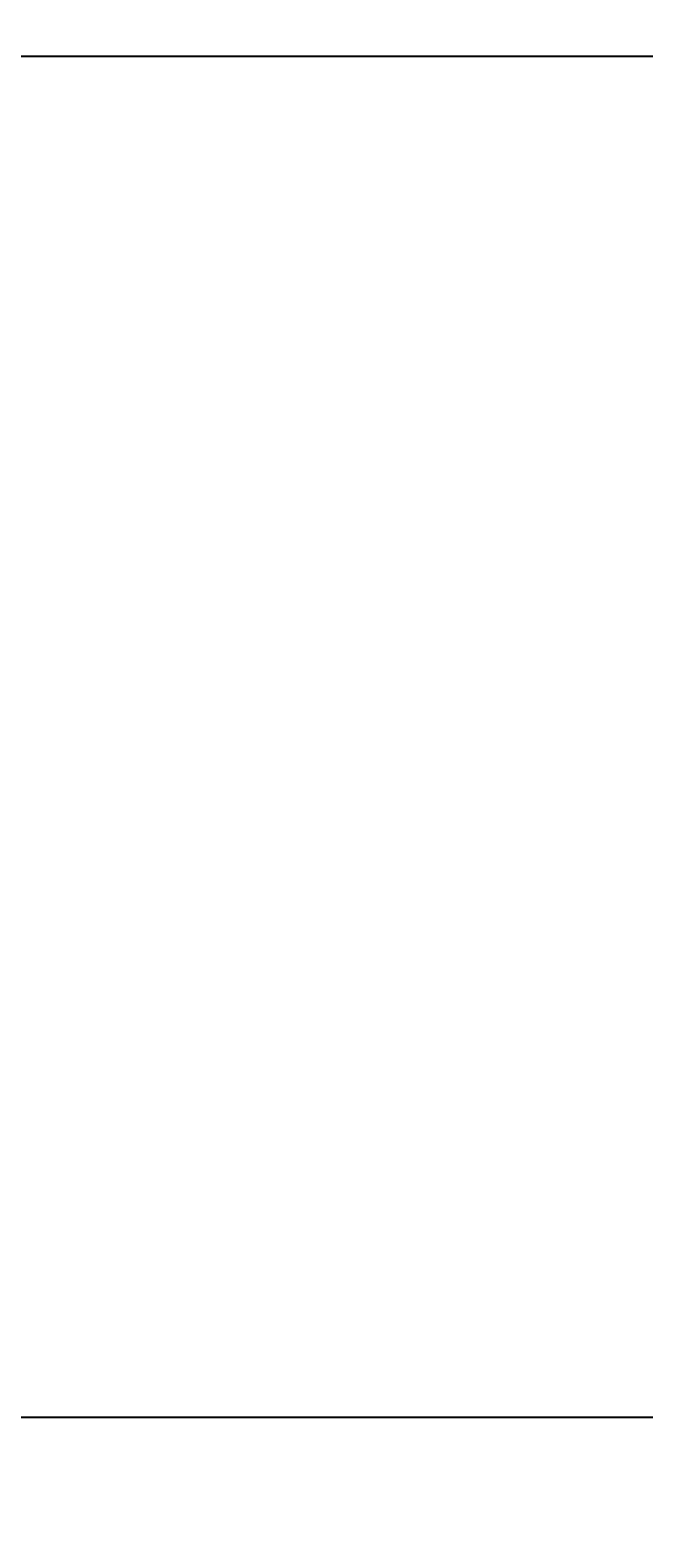
# Model space of a CAD drawing. Units: inches. Extents: x 35362 to 73946, y 43607 to 67532.
# Tile 19 of 134: x 48148 to 48340, y 46091 to 46564. Entities that reach past the tile are written whole.
import ezdxf

# ---------------------------------------------------------------- set-up
doc = ezdxf.new("R2010")
doc.units = ezdxf.units.IN
doc.header["$MEASUREMENT"] = 0
doc.layers.add('A-ANNO-DIMS', color=2, linetype='Continuous', lineweight=18)
doc.styles.get("Standard").update_dxf_attribs({"font": 'arial.ttf'})
doc.dimstyles.get("Standard").update_dxf_attribs({"dimtxt": 0.18, "dimasz": 0.18, "dimexe": 0.18, "dimexo": 0.0625, "dimgap": 0.09, "dimtad": 0, "dimtih": 1, "dimtoh": 1, "dimdec": 4, "dimzin": 0, "dimdsep": 46, "dimtxsty": 'Standard', "dimcen": 0.09, "dimadec": 0, "dimazin": 0, "dimtfac": 1, "dimtdec": 4, "dimtofl": 0, "dimtmove": 0, "dimatfit": 3, "dimfxl": 1, "dimtolj": 1, "dimtzin": 0, "dimarcsym": 0})

# ---------------------------------------------------------------- blocks, each defined once
blk = doc.blocks.new('*D5')
at = {"layer": 'A-ANNO-DIMS', "color": 0, "lineweight": -2, "transparency": 16777216}
for p, q in [((37121.95, 46919.32), (37121.95, 43606.68)), ((69871.5, 45449.83), (69871.5, 43606.68)), ((37122.13, 43606.86), (53496.29, 43606.86)), ((69871.32, 43606.86), (53497.15, 43606.86))]:
    blk.add_line(p, q, dxfattribs=at)
at = {"layer": 'A-ANNO-DIMS', "color": 0, "transparency": 16777216}
for points in [[(37122.13, 43606.89), (37122.13, 43606.83), (37121.95, 43606.86)], [(69871.32, 43606.89), (69871.32, 43606.83), (69871.5, 43606.86)]]:
    blk.add_solid(points, dxfattribs=at)
at = {"layer": 'Defpoints', "color": 0, "transparency": 16777216}
for p in [(37121.95, 46919.38), (69871.5, 45449.89), (69871.5, 43606.86)]:
    blk.add_point(p, dxfattribs=at)
at = {"layer": 'A-ANNO-DIMS', "color": 0, "transparency": 16777216, "insert": (53496.72, 43606.86), "char_height": 0.18, "attachment_point": 5}
blk.add_mtext('\\A1;32750', dxfattribs=at)
blk = doc.blocks.new('*D11')
at = {"layer": 'A-ANNO-DIMS', "color": 0, "lineweight": -2, "transparency": 16777216}
for p, q in [((47978.66, 56028.77), (47978.66, 43606.68)), ((53109.76, 56028.77), (53109.76, 43606.68)), ((47978.84, 43606.86), (50543.87, 43606.86)), ((53109.58, 43606.86), (50544.55, 43606.86))]:
    blk.add_line(p, q, dxfattribs=at)
at = {"layer": 'A-ANNO-DIMS', "color": 0, "transparency": 16777216}
for points in [[(47978.84, 43606.89), (47978.84, 43606.83), (47978.66, 43606.86)], [(53109.58, 43606.89), (53109.58, 43606.83), (53109.76, 43606.86)]]:
    blk.add_solid(points, dxfattribs=at)
at = {"layer": 'Defpoints', "color": 0, "transparency": 16777216}
for p in [(47978.66, 56028.84), (53109.76, 56028.84), (53109.76, 43606.86)]:
    blk.add_point(p, dxfattribs=at)
at = {"layer": 'A-ANNO-DIMS', "color": 0, "transparency": 16777216, "insert": (50544.21, 43606.86), "char_height": 0.18, "attachment_point": 5}
blk.add_mtext('\\A1;5131', dxfattribs=at)
blk = doc.blocks.new('*D27')
at = {"layer": 'A-ANNO-DIMS', "color": 0, "lineweight": -2, "transparency": 16777216}
for p, q in [((47978.66, 56028.77), (47978.66, 43606.68)), ((48373.49, 53428.96), (48373.49, 43606.68)), ((47978.84, 43606.86), (48175.68, 43606.86)), ((48373.31, 43606.86), (48176.47, 43606.86))]:
    blk.add_line(p, q, dxfattribs=at)
at = {"layer": 'A-ANNO-DIMS', "color": 0, "transparency": 16777216}
for points in [[(47978.84, 43606.89), (47978.84, 43606.83), (47978.66, 43606.86)], [(48373.31, 43606.89), (48373.31, 43606.83), (48373.49, 43606.86)]]:
    blk.add_solid(points, dxfattribs=at)
at = {"layer": 'Defpoints', "color": 0, "transparency": 16777216}
for p in [(47978.66, 56028.84), (48373.49, 53429.02), (48373.49, 43606.86)]:
    blk.add_point(p, dxfattribs=at)
at = {"layer": 'A-ANNO-DIMS', "color": 0, "transparency": 16777216, "insert": (48176.08, 43606.86), "char_height": 0.18, "attachment_point": 5}
blk.add_mtext('\\A1;394.8', dxfattribs=at)
blk = doc.blocks.new('*D67')
at = {"layer": 'A-ANNO-DIMS', "color": 0, "lineweight": -2, "transparency": 16777216}
for p, q in [((56873.54, 53351.53), (35361.77, 53351.53)), ((35361.95, 53351.35), (35361.95, 49400.89)), ((35361.95, 45450.07), (35361.95, 49400.53)), ((53793.58, 45449.89), (35361.77, 45449.89))]:
    blk.add_line(p, q, dxfattribs=at)
at = {"layer": 'A-ANNO-DIMS', "color": 0, "transparency": 16777216}
for points in [[(35361.92, 53351.35), (35361.98, 53351.35), (35361.95, 53351.53)], [(35361.92, 45450.07), (35361.98, 45450.07), (35361.95, 45449.89)]]:
    blk.add_solid(points, dxfattribs=at)
at = {"layer": 'Defpoints', "color": 0, "transparency": 16777216}
for p in [(35361.95, 53351.53), (56873.6, 53351.53), (53793.64, 45449.89)]:
    blk.add_point(p, dxfattribs=at)
at = {"layer": 'A-ANNO-DIMS', "color": 0, "transparency": 16777216, "insert": (35361.95, 49400.71), "char_height": 0.18, "attachment_point": 5}
blk.add_mtext('\\A1;7901.6', dxfattribs=at)
blk = doc.blocks.new('*D76')
at = {"layer": 'A-ANNO-DIMS', "color": 0, "lineweight": -2, "transparency": 16777216}
for p, q in [((54052.84, 46555.29), (35361.77, 46555.29)), ((35361.95, 46555.11), (35361.95, 46342.27)), ((35361.95, 46129.06), (35361.95, 46341.9)), ((53793.58, 46128.88), (35361.77, 46128.88))]:
    blk.add_line(p, q, dxfattribs=at)
at = {"layer": 'A-ANNO-DIMS', "color": 0, "transparency": 16777216}
for points in [[(35361.92, 46555.11), (35361.98, 46555.11), (35361.95, 46555.29)], [(35361.92, 46129.06), (35361.98, 46129.06), (35361.95, 46128.88)]]:
    blk.add_solid(points, dxfattribs=at)
at = {"layer": 'Defpoints', "color": 0, "transparency": 16777216}
for p in [(35361.95, 46555.29), (54052.9, 46555.29), (53793.64, 46128.88)]:
    blk.add_point(p, dxfattribs=at)
at = {"layer": 'A-ANNO-DIMS', "color": 0, "transparency": 16777216, "insert": (35361.95, 46342.09), "char_height": 0.18, "attachment_point": 5}
blk.add_mtext('\\A1;426.4', dxfattribs=at)
blk = doc.blocks.new('*D90')
at = {"layer": 'A-ANNO-DIMS', "color": 0, "lineweight": -2, "transparency": 16777216}
for p, q in [((53707.72, 47291.29), (35361.77, 47291.29)), ((35361.95, 47291.11), (35361.95, 46710.26)), ((35361.95, 46129.06), (35361.95, 46709.9)), ((53793.58, 46128.88), (35361.77, 46128.88))]:
    blk.add_line(p, q, dxfattribs=at)
at = {"layer": 'A-ANNO-DIMS', "color": 0, "transparency": 16777216}
for points in [[(35361.92, 47291.11), (35361.98, 47291.11), (35361.95, 47291.29)], [(35361.92, 46129.06), (35361.98, 46129.06), (35361.95, 46128.88)]]:
    blk.add_solid(points, dxfattribs=at)
at = {"layer": 'Defpoints', "color": 0, "transparency": 16777216}
for p in [(53707.78, 47291.29), (35361.95, 46128.88), (53793.64, 46128.88)]:
    blk.add_point(p, dxfattribs=at)
at = {"layer": 'A-ANNO-DIMS', "color": 0, "transparency": 16777216, "insert": (35361.95, 46710.08), "char_height": 0.18, "attachment_point": 5}
blk.add_mtext('\\A1;1162.4', dxfattribs=at)

msp = doc.modelspace()

# ---------------------------------------------------------------- dimensions: what is measured, and where the dimension line sits
at = {"layer": 'A-ANNO-DIMS'}
for base, p1, p2, override, picture, middle in [((53109.76, 43606.859), (47978.665, 56028.836), (53109.76, 56028.836), {"dimdec": 0, "dimlfac": 1, "dimrnd": 0, "dimzin": 0, "dimdsep": 46, "dimlunit": 2}, '*D11', (50544.212, 43606.859)), ((48373.492, 43606.859), (47978.665, 56028.836), (48373.492, 53429.019), {"dimdec": 1, "dimlfac": 1, "dimrnd": 0, "dimzin": 0, "dimdsep": 46, "dimlunit": 2}, '*D27', (48176.078, 43606.859)), ((69871.496, 43606.859), (37121.949, 46919.381), (69871.496, 45449.894), {"dimdec": 0, "dimlfac": 1, "dimrnd": 0, "dimzin": 0, "dimdsep": 46, "dimlunit": 2}, '*D5', (53496.723, 43606.859))]:
    dim = msp.add_linear_dim(base=base, p1=p1, p2=p2, dimstyle='Standard', override=override, dxfattribs=at)
    dim.commit()
    dim.dimension.update_dxf_attribs({"geometry": picture, "text_midpoint": middle})
for base, p1, p2, picture, middle in [((35361.949, 53351.529), (53793.638, 45449.894), (56873.602, 53351.529), '*D67', (35361.949, 49400.712)), ((35361.949, 46128.878), (53707.781, 47291.285), (53793.638, 46128.878), '*D90', (35361.949, 46710.081)), ((35361.949, 46555.293), (53793.638, 46128.878), (54052.899, 46555.293), '*D76', (35361.949, 46342.086))]:
    dim = msp.add_linear_dim(base=base, p1=p1, p2=p2, angle=90, dimstyle='Standard', override={"dimdec": 1, "dimlfac": 1, "dimrnd": 0, "dimzin": 0, "dimdsep": 46, "dimlunit": 2}, dxfattribs=at)
    dim.commit()
    dim.dimension.update_dxf_attribs({"geometry": picture, "text_midpoint": middle})

doc.saveas('drawing.dxf')
